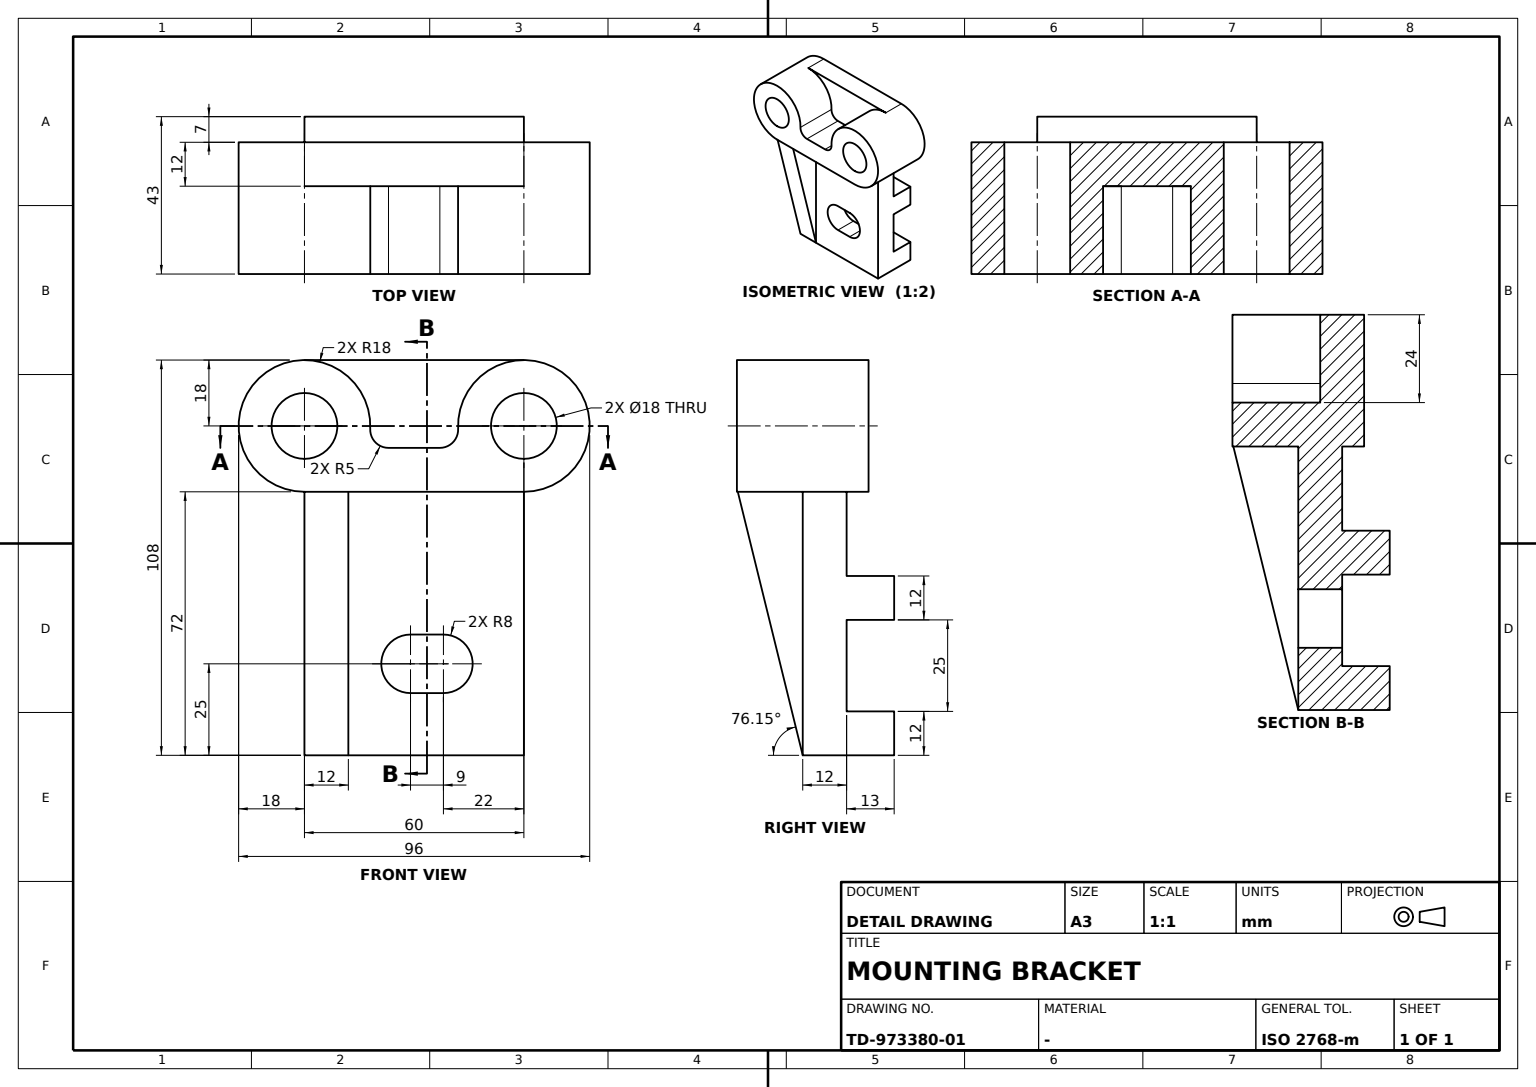
CATIA V5 part; units mm, degrees
sketch "Sketch1" plane through (0, 0, 0) normal (0, 1, 0) x (-1, 0, 0)
  point P0 (0, -36)
  line L0 (0, -36) -> (0, 36)
  line L1 (0, 36) -> (12, 36)
  line L2 (12, 36) -> (12, 13)
  line L3 (12, 13) -> (25, 13)
  line L4 (25, 13) -> (25, 1)
  line L5 (25, 1) -> (12, 1)
  point P1 (12, 1)
  line L6 (12, 1) -> (12, -24)
  line L7 (12, -24) -> (25, -24)
  line L8 (25, -24) -> (25, -36)
  line L9 (25, -36) -> (0, -36)
  dimension "length L8" = 12
  dimension "length L9" = 25
  dimension "distance L0 L2" = 12
  dimension "length L4" = 12
  dimension "distance L7 L5" = 25
  dimension "length L5" = 13
  dimension "length L0" = 72
  constraint coincidence P0 y-axis
  constraint coincidence P1 L2
  constraint vertical L0 y-axis
  constraint vertical L2 y-axis
  constraint vertical L4 y-axis
  constraint vertical L6 y-axis
  constraint vertical L8 y-axis
  constraint horizontal L1 x-axis
  constraint horizontal L3 x-axis
  constraint horizontal L5 x-axis
  constraint horizontal L7 x-axis
  constraint horizontal L9 x-axis
  constraint symmetry L9 L1 x-axis
extrude "Pad1" add sketch "Sketch1" along normal mid plane 60
sketch "Sketch2" plane through (0, 0, 0) normal (1, 0, 0) x (0, 1, 0)
  arc A0 (-13.0294, 48) -> (-30, 36) centre (-30, 54) ccw
  point P0 (-30, 54)
  arc A1 (30, 36) -> (13.0294, 48) centre (30, 54) ccw
  point P1 (30, 54)
  circle A2 centre (30, 54) radius 9
  circle A3 centre (-30, 54) radius 9
  line L0 (-13.0294, 48) -> (13.0294, 48)
  line L1 (-30, 36) -> (30, 36)
  line L2 (-30, 36) -> (30, 36) construction
  dimension "radius A2" = 9
  dimension "radius A3" = 9
  dimension "distance L0 L1" = 12
  dimension "radius A0" = 18
  dimension "length L1" = 60
  constraint horizontal L0 x-axis
  constraint horizontal L1 x-axis
  constraint symmetry P0 P1 y-axis
  constraint tangency L1 A0
  constraint tangency L1 A1
  constraint coincidence L1 L2
extrude "Pad2" add sketch "Sketch2" along normal mid plane 36
fillet "Fillet1" radius 5 2 edges at (0, -13.0294, 48) (0, 13.0294, 48)
sketch "Sketch3" plane through (-18, 0, 0) normal (-1, 0, 0) x (0, -1, 0)
  point P0 (-30, 72)
  line L0 (-30, 72) -> (30, 72)
  point P1 (30, 72)
  arc A0 (30, 36) -> (13.0294, 48) centre (30, 54) ccw construction
  arc A1 (-13.0294, 48) -> (-30, 36) centre (-30, 54) ccw construction
  arc A2 (-13.0294, 48) -> (-30, 36) centre (-30, 54) ccw construction
  arc A3 (30, 36) -> (13.0294, 48) centre (30, 54) ccw construction
  arc A4 (30, 72) -> (12.017, 53.2174) centre (30, 54) ccw
  point P2 (12.017, 53.2174)
  line L1 (-7.0217, 48) -> (7.0217, 48)
  arc A5 (7.0217, 48) -> (12.017, 53.2174) centre (7.0217, 53) ccw
  point P3 (12.017, 53.2174)
  arc A6 (-12.017, 53.2174) -> (-30, 72) centre (-30, 54) ccw
  point P4 (-12.017, 53.2174)
  arc A7 (-12.017, 53.2174) -> (-7.0217, 48) centre (-7.0217, 53) ccw
  point P5 (-12.017, 53.2174)
  constraint horizontal L0 x-axis
  constraint coincidence P1 A0
  constraint coincidence P0 A1
  constraint coincidence P2 P3
  constraint coincidence P4 P5
  constraint tangency L0 A2
  constraint tangency L0 A3
extrude "Pad3" add sketch "Sketch3" against normal blind 12
sketch "Sketch4" plane through (0, -30, 0) normal (0, -1, 0) x (1, 0, 0)
  line L0 (0, 37) -> (18, 37)
  line L1 (18, 37) -> (0, -36)
  point P0 (0, -36)
  line L2 (0, -36) -> (0, 37)
  line L3 (0, 36) -> (0, -36) construction
  line L4 (0, -36) -> (-25, -36) construction
  dimension "length L2" = 73
  dimension "length L0" = 18
  constraint horizontal L0 x-axis
  constraint vertical L2 y-axis
  constraint coincidence L2 L3
  constraint coincidence P0 L4
extrude "Pad4" add sketch "Sketch4" against normal blind 12
sketch "Sketch5" plane through (0, 0, 0) normal (1, 0, 0) x (0, 1, 0)
  arc A0 (-1, -3) -> (-1, -19) centre (-1, -11) ccw
  point P0 (-1, -11)
  arc A1 (8, -19) -> (8, -3) centre (8, -11) ccw
  point P1 (8, -11)
  line L0 (-30, -36) -> (30, -36) construction
  line L1 (-30, -36) -> (30, -36) construction
  line L2 (-1, -3) -> (8, -3)
  line L3 (30, 36) -> (30, -36) construction
  line L4 (-1, -19) -> (8, -19)
  dimension "radius A0" = 8
  dimension "distance P1 L0" = 25
  dimension "distance P0 L1" = 25
  dimension "length L2" = 9
  dimension "distance P1 L3" = 22
  constraint horizontal L2 x-axis
  constraint horizontal L4 x-axis
  constraint tangency L2 A1
  constraint tangency L2 A0
  constraint tangency L4 A1
extrude "Pocket1" cut sketch "Sketch5" against normal through all
